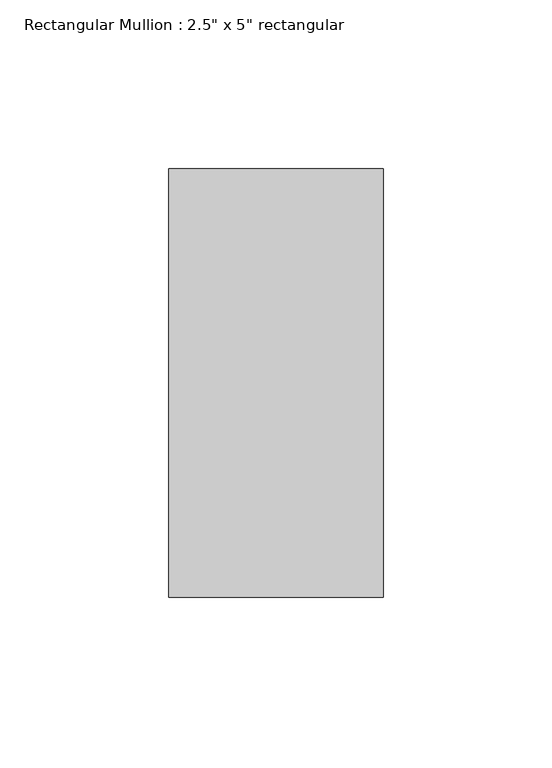
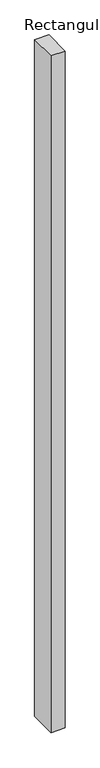
"""IFC4 building model written with IfcOpenShell, lengths in millimetres: member geometry."""

from ifc_helpers import new_model, si_unit, frame, origin, place, context, project, spatial, polyline, outline, extrude, source, transform, mapped, element, save


def member_01255749(model_context):
    return source(origin(), model_context, "Body", "SweptSolid", [
        extrude(outline(polyline([(0.0, 63.5), (0.0, -63.5), (-63.5, -63.5), (-63.5, 63.5), (0.0, 63.5)])), frame((0.0, 0.0, -3213.1), z_axis=(0.0, 0.0, 1.0), x_axis=(1.0, 0.0, 0.0)), (0.0, 0.0, 1.0), 3213.1),
    ])


if __name__ == "__main__":
    model = new_model("IFC4")
    model_context = context("Model", 3, world=origin())
    ifc_project = project(units=[si_unit("LENGTHUNIT", "METRE", prefix="MILLI")], contexts=[model_context])
    site = spatial("IfcSite", under=ifc_project)
    building = spatial("IfcBuilding", under=site)
    placement = place(None, origin())
    member_shape = member_01255749(model_context)
    element("IfcMember", 1, ObjectType="Rectangular Mullion : 2.5\" x 5\" rectangular", at=placement, inside=building, context=model_context, shape_type="MappedRepresentation", body=[
        mapped(member_shape, transform((0.0, 0.0, 0.0), x_axis=(1.0, 0.0, 0.0), y_axis=(0.0, 1.0, 0.0), z_axis=(0.0, 0.0, 1.0))),
    ])
    save(model, "model.ifc")

# Revit data of these elements
# Type "Rectangular Mullion : 2.5\" x 5\" rectangular"
#   built-in parameter 1007304 = 0.416667 (stored number, unit not read)
#   built-in parameter 1007301 = 0.104167 (stored number, unit not read)
#   built-in parameter 1007300 = 0.104167 (stored number, unit not read)
# Element 1 (IfcMember, "Rectangular Mullion : 2.5\" x 5\" rectangular")
#   Materials on its faces: "Aluminum"
# Materials
#   "Aluminum": class "Metal", colour RGB 247 247 247, transparency 0, Description = "Aluminum 6061", Cost = 0
